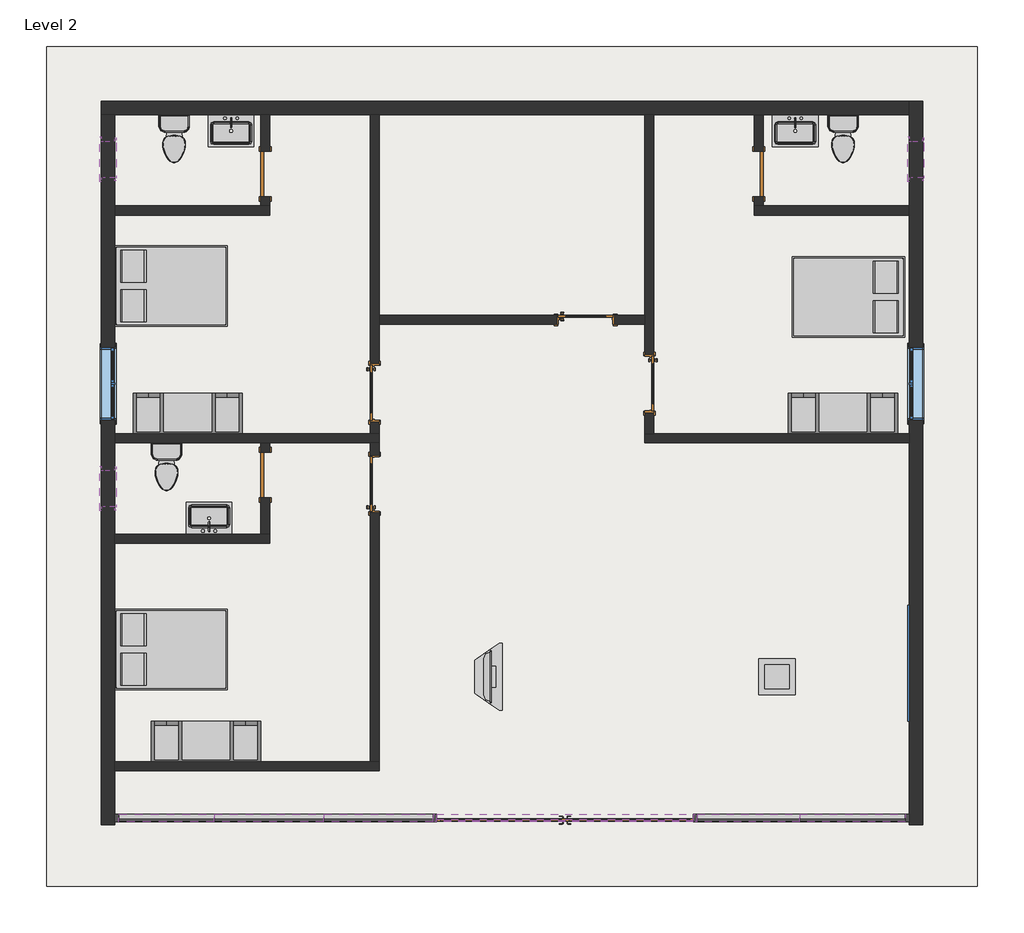
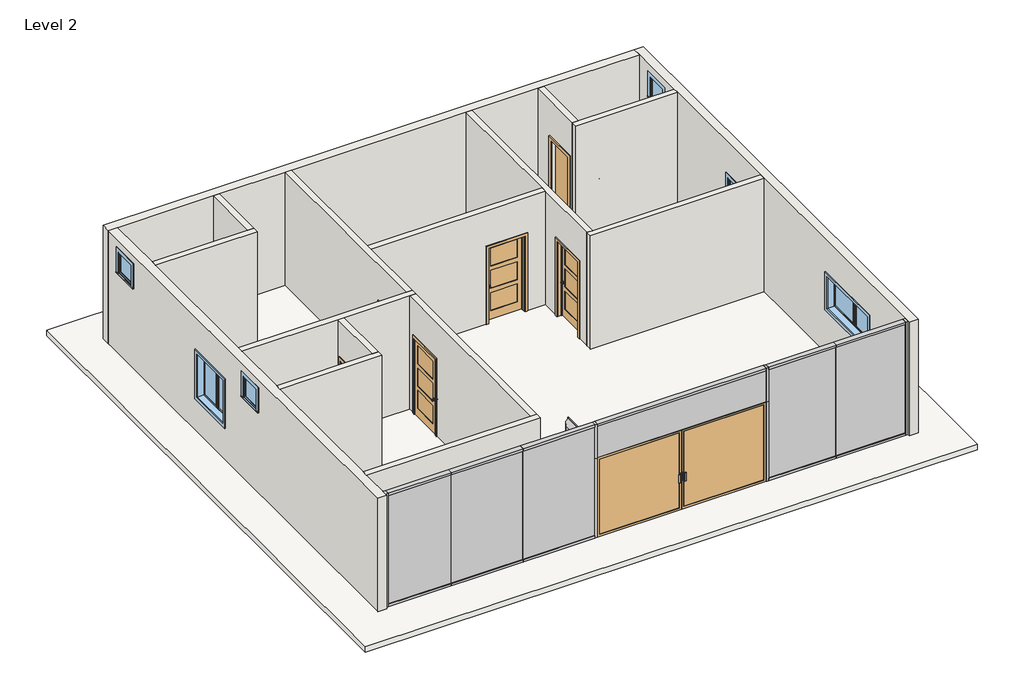
# One storey, incomplete: 17 members, 16 walls, 9 furniture elements, 8 doors, 6 flow terminals, 6 plates, 6 windows, 1 slab.
"""IFC4 building model written with IfcOpenShell, lengths in millimetres."""

from ifc_helpers import new_model, si_unit, frame, origin, place, context, project, spatial, polyline, outline, extrude, faceted_brep, transform, mapped, element, save
from components import door_curtain_wall_double_storefront_door_curtain_wall_double_6e8ba87c, door_ac27962c, door_c5233792, door_d64d7266, door_c31ea698, flow_terminal_38af2918, toilet_domestic_3d_toilet_domestic_3d_f7549cf7, toilet_domestic_3d_toilet_domestic_3d_183bbd19, furniture_c8abb964, furniture_cf0b6580, furniture_56245f3a, tv_stand_tv_stand_94947415, furniture_b5c51a22, member_3f395ae9, member_d9503739, member_2fae0574, member_2501c824, member_6d5c3e5e, member_4da692ab, member_3374d9b6, member_73c23c35, system_panel_glazed_a38948d3, system_panel_glazed_97c7e3fb, system_panel_glazed_baea53c3, system_panel_glazed_5d99744d, system_panel_glazed_41d8189d, window_534dcd48, window_6788402d, window_3ed046d9

model = new_model("IFC4")

# Units and contexts
model_context = context("Model", 3, world=origin())
ifc_project = project(units=[si_unit("LENGTHUNIT", "METRE", prefix="MILLI")], contexts=[model_context])

# Site, building, storey
site = spatial("IfcSite", under=ifc_project)
building = spatial("IfcBuilding", under=site)
storey = spatial("IfcBuildingStorey", under=building, Name="Level 2", Elevation=3048.0)

# Doors
placement = place(None, origin())
door_curtain_wall_double_storefront_door_curtain_wall_double_shape = door_curtain_wall_double_storefront_door_curtain_wall_double_6e8ba87c(model_context)
element("IfcDoor", 1, ObjectType="Door-Curtain-Wall-Double-Storefront : Door-Curtain-Wall-Double-Storefront", at=placement, inside=storey, context=model_context, shape_type="MappedRepresentation", body=[
    mapped(door_curtain_wall_double_storefront_door_curtain_wall_double_shape, transform((-6799.0866603, -9419.3331121, 3048.0), x_axis=(-1.0, 0.0, 0.0), y_axis=(0.0, -1.0, 0.0), z_axis=(0.0, 0.0, 1.0))),
])
door_shape = door_ac27962c(model_context)
element("IfcDoor", 2, ObjectType="Door-Interior-Single-3_Panel_Vert-Wood : 36\" x 80\"", at=placement, inside=storey, context=model_context, shape_type="MappedRepresentation", body=[
    mapped(door_shape, transform((-9989.9616603, -3831.3331121, 3048.0), x_axis=(0.0, 1.0, 0.0), y_axis=(-1.0, 0.0, 0.0), z_axis=(0.0, 0.0, 1.0))),
])
element("IfcDoor", 3, ObjectType="Door-Interior-Single-3_Panel_Vert-Wood : 36\" x 80\"", at=placement, inside=storey, context=model_context, shape_type="MappedRepresentation", body=[
    mapped(door_shape, transform((-5386.2116603, -2154.9331121, 3048.0), x_axis=(0.0, -1.0, 0.0), y_axis=(1.0, 0.0, 0.0), z_axis=(0.0, 0.0, 1.0))),
])
element("IfcDoor", 4, ObjectType="Door-Interior-Single-3_Panel_Vert-Wood : 36\" x 80\"", at=placement, inside=storey, context=model_context, shape_type="MappedRepresentation", body=[
    mapped(door_shape, transform((-6456.1866603, -1084.9581121, 3048.0), x_axis=(1.0, 0.0, 0.0), y_axis=(0.0, 1.0, 0.0), z_axis=(0.0, 0.0, 1.0))),
])
door_2_shape = door_c5233792(model_context)
element("IfcDoor", 5, ObjectType="Door-Interior-Single-3_Panel_Vert-Wood : 36\" x 80\"", at=placement, inside=storey, context=model_context, shape_type="MappedRepresentation", body=[
    mapped(door_2_shape, transform((-9989.9616603, -2307.3331121, 3048.0), x_axis=(0.0, -1.0, 0.0), y_axis=(1.0, 0.0, 0.0), z_axis=(0.0, 0.0, 1.0))),
])
door_3_shape = door_d64d7266(model_context)
element("IfcDoor", 6, ObjectType="Door-Single-Panel : 30\" x 80\"", at=placement, inside=storey, context=model_context, shape_type="MappedRepresentation", body=[
    mapped(door_3_shape, transform((-11815.5866603, 1350.2668879, 3048.0), x_axis=(0.0, -1.0, 0.0), y_axis=(1.0, 0.0, 0.0), z_axis=(0.0, 0.0, 1.0))),
])
door_4_shape = door_c31ea698(model_context)
element("IfcDoor", 7, ObjectType="Door-Single-Panel : 30\" x 80\"", at=placement, inside=storey, context=model_context, shape_type="MappedRepresentation", body=[
    mapped(door_4_shape, transform((-11815.5866603, -3678.9331121, 3048.0), x_axis=(0.0, 1.0, 0.0), y_axis=(-1.0, 0.0, 0.0), z_axis=(0.0, 0.0, 1.0))),
])
element("IfcDoor", 8, ObjectType="Door-Single-Panel : 30\" x 80\"", at=placement, inside=storey, context=model_context, shape_type="MappedRepresentation", body=[
    mapped(door_4_shape, transform((-3560.5866603, 1350.2668879, 3048.0), x_axis=(0.0, -1.0, 0.0), y_axis=(1.0, 0.0, 0.0), z_axis=(0.0, 0.0, 1.0))),
])

# Flow terminals
flow_terminal_shape = flow_terminal_38af2918(model_context)
element("IfcFlowTerminal", 9, ObjectType="Sink Kitchen-Single : 30\" x 21\"", at=placement, inside=storey, context=model_context, shape_type="MappedRepresentation", body=[
    mapped(flow_terminal_shape, transform((-12402.7759008, 2071.8214868, 3048.0), x_axis=(1.0, 0.0, 0.0), y_axis=(0.0, 1.0, 0.0), z_axis=(0.0, 0.0, 1.0))),
])
element("IfcFlowTerminal", 10, ObjectType="Sink Kitchen-Single : 30\" x 21\"", at=placement, inside=storey, context=model_context, shape_type="MappedRepresentation", body=[
    mapped(flow_terminal_shape, transform((-2966.6759008, 2071.8214868, 3048.0), x_axis=(1.0000000000000002, 0.0, 0.0), y_axis=(0.0, 1.0000000000000002, 0.0), z_axis=(0.0, 0.0, 1.0))),
])
element("IfcFlowTerminal", 11, ObjectType="Sink Kitchen-Single : 30\" x 21\"", at=placement, inside=storey, context=model_context, shape_type="MappedRepresentation", body=[
    mapped(flow_terminal_shape, transform((-12739.6974197, -4406.8377109, 3048.0), x_axis=(-1.0000000000000002, 0.0, 0.0), y_axis=(0.0, -1.0000000000000002, 0.0), z_axis=(0.0, 0.0, 1.0))),
])
toilet_domestic_3d_toilet_domestic_3d_shape = toilet_domestic_3d_toilet_domestic_3d_f7549cf7(model_context)
toilet_domestic_3d_toilet_domestic_3d_2_shape = toilet_domestic_3d_toilet_domestic_3d_183bbd19(model_context)
element("IfcFlowTerminal", 12, ObjectType="Toilet-Domestic-3D : Toilet-Domestic-3D", at=placement, inside=storey, context=model_context, shape_type="MappedRepresentation", body=[
    mapped(toilet_domestic_3d_toilet_domestic_3d_shape, transform((-13339.5866603, 1846.1708606, 3048.0), x_axis=(1.0000000000000007, 0.0, 0.0), y_axis=(0.0, 1.0000000000000007, 0.0), z_axis=(0.0, 0.0, 1.0))),
    mapped(toilet_domestic_3d_toilet_domestic_3d_2_shape, transform((-13339.5866603, 1846.1708606, 3048.0), x_axis=(1.0000000000000007, 0.0, 0.0), y_axis=(0.0, 1.0000000000000007, 0.0), z_axis=(0.0, 0.0, 1.0))),
])
element("IfcFlowTerminal", 13, ObjectType="Toilet-Domestic-3D : Toilet-Domestic-3D", at=placement, inside=storey, context=model_context, shape_type="MappedRepresentation", body=[
    mapped(toilet_domestic_3d_toilet_domestic_3d_shape, transform((-2150.8866603, 1846.1708606, 3048.0), x_axis=(1.0, 0.0, 0.0), y_axis=(0.0, 1.0, 0.0), z_axis=(0.0, 0.0, 1.0))),
    mapped(toilet_domestic_3d_toilet_domestic_3d_2_shape, transform((-2150.8866603, 1846.1708606, 3048.0), x_axis=(1.0, 0.0, 0.0), y_axis=(0.0, 1.0, 0.0), z_axis=(0.0, 0.0, 1.0))),
])
element("IfcFlowTerminal", 14, ObjectType="Toilet-Domestic-3D : Toilet-Domestic-3D", at=placement, inside=storey, context=model_context, shape_type="MappedRepresentation", body=[
    mapped(toilet_domestic_3d_toilet_domestic_3d_shape, transform((-13466.5866603, -3640.2291394, 3048.0), x_axis=(1.0, 0.0, 0.0), y_axis=(0.0, 1.0, 0.0), z_axis=(0.0, 0.0, 1.0))),
    mapped(toilet_domestic_3d_toilet_domestic_3d_2_shape, transform((-13466.5866603, -3640.2291394, 3048.0), x_axis=(1.0, 0.0, 0.0), y_axis=(0.0, 1.0, 0.0), z_axis=(0.0, 0.0, 1.0))),
])

# Furniture
furniture_shape = furniture_c8abb964(model_context)
element("IfcFurniture", 15, ObjectType="Bed-Box : Double 53\" x 74\"", at=placement, inside=storey, context=model_context, shape_type="MappedRepresentation", body=[
    mapped(furniture_shape, transform((-13624.8161685, -859.5331121, 3048.0), x_axis=(0.0, 1.0, 0.0), y_axis=(-1.0, 0.0, 0.0), z_axis=(0.0, 0.0, 1.0))),
])
element("IfcFurniture", 16, ObjectType="Bed-Box : Double 53\" x 74\"", at=placement, inside=storey, context=model_context, shape_type="MappedRepresentation", body=[
    mapped(furniture_shape, transform((-13624.8161685, -6939.0855711, 3048.0), x_axis=(0.0, 1.0000000000000002, 0.0), y_axis=(-1.0000000000000002, 0.0, 0.0), z_axis=(0.0, 0.0, 1.0))),
])
element("IfcFurniture", 17, ObjectType="Bed-Box : Double 53\" x 74\"", at=placement, inside=storey, context=model_context, shape_type="MappedRepresentation", body=[
    mapped(furniture_shape, transform((-1827.5571521, -367.980653, 3048.0), x_axis=(0.0, -1.0, 0.0), y_axis=(1.0, 0.0, 0.0), z_axis=(0.0, 0.0, 1.0))),
])
furniture_2_shape = furniture_cf0b6580(model_context)
element("IfcFurniture", 18, ObjectType="Entertainment Center : 72\" x 72\" x 24\"", at=placement, inside=storey, context=model_context, shape_type="MappedRepresentation", body=[
    mapped(furniture_2_shape, transform((-2150.8866603, -3094.7331121, 3048.0), x_axis=(-1.0000000000000002, 0.0, 0.0), y_axis=(0.0, -1.0000000000000002, 0.0), z_axis=(0.0, 0.0, 1.0))),
])
element("IfcFurniture", 19, ObjectType="Entertainment Center : 72\" x 72\" x 24\"", at=placement, inside=storey, context=model_context, shape_type="MappedRepresentation", body=[
    mapped(furniture_2_shape, transform((-13110.9866603, -3094.7331121, 3048.0), x_axis=(-1.0, 0.0, 0.0), y_axis=(0.0, -1.0, 0.0), z_axis=(0.0, 0.0, 1.0))),
])
element("IfcFurniture", 20, ObjectType="Entertainment Center : 72\" x 72\" x 24\"", at=placement, inside=storey, context=model_context, shape_type="MappedRepresentation", body=[
    mapped(furniture_2_shape, transform((-12806.1866603, -8581.1331121, 3048.0), x_axis=(-1.0, 0.0, 0.0), y_axis=(0.0, -1.0, 0.0), z_axis=(0.0, 0.0, 1.0))),
])
furniture_3_shape = furniture_56245f3a(model_context)
element("IfcFurniture", 21, ObjectType="TV - Flat Screen : 32\"", at=placement, inside=storey, context=model_context, shape_type="MappedRepresentation", body=[
    mapped(furniture_3_shape, transform((-8100.8328523, -7053.1885979, 3657.6), x_axis=(0.0, 1.0000000000000002, 0.0), y_axis=(-1.0000000000000002, 0.0, 0.0), z_axis=(0.0, 0.0, 1.0))),
])
tv_stand_tv_stand_shape = tv_stand_tv_stand_94947415(model_context)
element("IfcFurniture", 22, ObjectType="TV Stand : TV Stand", at=placement, inside=storey, context=model_context, shape_type="MappedRepresentation", body=[
    mapped(tv_stand_tv_stand_shape, transform((-8310.3866603, -7182.3211141, 3048.0), x_axis=(0.0, 1.0000000000000002, 0.0), y_axis=(-1.0000000000000002, 0.0, 0.0), z_axis=(0.0, 0.0, 1.0))),
])
furniture_4_shape = furniture_b5c51a22(model_context)
element("IfcFurniture", 23, ObjectType="Table-Coffee : 24\" x 24\" x 24\"", at=placement, inside=storey, context=model_context, shape_type="MappedRepresentation", body=[
    mapped(furniture_4_shape, transform((-3274.0524269, -7152.3441899, 3048.0), x_axis=(1.0, 0.0, 0.0), y_axis=(0.0, 1.0, 0.0), z_axis=(0.0, 0.0, 1.0))),
])

# Members
member_shape = member_3f395ae9(model_context)
element("IfcMember", 24, ObjectType="Rectangular Mullion : 2.5\" x 5\" rectangular", at=placement, inside=storey, context=model_context, shape_type="MappedRepresentation", body=[
    mapped(member_shape, transform((-14330.1866603, -9419.3331121, 3048.0), x_axis=(-1.0, 0.0, 0.0), y_axis=(0.0, 1.0, 0.0), z_axis=(0.0, 0.0, -1.0))),
])
member_2_shape = member_d9503739(model_context)
element("IfcMember", 25, ObjectType="Rectangular Mullion : 2.5\" x 5\" rectangular", at=placement, inside=storey, context=model_context, shape_type="MappedRepresentation", body=[
    mapped(member_2_shape, transform((-14266.6866603, -9419.3331121, 6096.0), x_axis=(0.0, 0.0, 1.0), y_axis=(0.0, 1.0, 0.0), z_axis=(-1.0, 0.0, 0.0))),
])
member_3_shape = member_2fae0574(model_context)
element("IfcMember", 26, ObjectType="Rectangular Mullion : 2.5\" x 5\" rectangular", at=placement, inside=storey, context=model_context, shape_type="MappedRepresentation", body=[
    mapped(member_3_shape, transform((-12666.4866603, -9419.3331121, 6096.0), x_axis=(0.0, 0.0, 1.0), y_axis=(0.0, 1.0, 0.0), z_axis=(-1.0, 0.0, 0.0))),
])
element("IfcMember", 27, ObjectType="Rectangular Mullion : 2.5\" x 5\" rectangular", at=placement, inside=storey, context=model_context, shape_type="MappedRepresentation", body=[
    mapped(member_2_shape, transform((-12666.4866603, -9419.3331121, 3048.0), x_axis=(0.0, 0.0, -1.0), y_axis=(0.0, 1.0, 0.0), z_axis=(1.0, 0.0, 0.0))),
])
element("IfcMember", 28, ObjectType="Rectangular Mullion : 2.5\" x 5\" rectangular", at=placement, inside=storey, context=model_context, shape_type="MappedRepresentation", body=[
    mapped(member_3_shape, transform((-9008.8866603, -9419.3331121, 3048.0), x_axis=(0.0, 0.0, -1.0), y_axis=(0.0, 1.0, 0.0), z_axis=(1.0, 0.0, 0.0))),
])
element("IfcMember", 29, ObjectType="Rectangular Mullion : 2.5\" x 5\" rectangular", at=placement, inside=storey, context=model_context, shape_type="MappedRepresentation", body=[
    mapped(member_3_shape, transform((-10837.6866603, -9419.3331121, 3048.0), x_axis=(0.0, 0.0, -1.0), y_axis=(0.0, 1.0, 0.0), z_axis=(1.0, 0.0, 0.0))),
])
member_4_shape = member_2501c824(model_context)
element("IfcMember", 30, ObjectType="Rectangular Mullion : 2.5\" x 5\" rectangular", at=placement, inside=storey, context=model_context, shape_type="MappedRepresentation", body=[
    mapped(member_4_shape, transform((-2874.7866603, -9419.3331121, 3048.0), x_axis=(0.0, 0.0, -1.0), y_axis=(0.0, 1.0, 0.0), z_axis=(1.0, 0.0, 0.0))),
])
member_5_shape = member_6d5c3e5e(model_context)
element("IfcMember", 31, ObjectType="Rectangular Mullion : 2.5\" x 5\" rectangular", at=placement, inside=storey, context=model_context, shape_type="MappedRepresentation", body=[
    mapped(member_5_shape, transform((-2874.7866603, -9419.3331121, 6096.0), x_axis=(0.0, 0.0, 1.0), y_axis=(0.0, 1.0, 0.0), z_axis=(-1.0, 0.0, 0.0))),
])
element("IfcMember", 32, ObjectType="Rectangular Mullion : 2.5\" x 5\" rectangular", at=placement, inside=storey, context=model_context, shape_type="MappedRepresentation", body=[
    mapped(member_5_shape, transform((-1109.4866603, -9419.3331121, 3048.0), x_axis=(0.0, 0.0, -1.0), y_axis=(0.0, 1.0, 0.0), z_axis=(1.0, 0.0, 0.0))),
])
element("IfcMember", 33, ObjectType="Rectangular Mullion : 2.5\" x 5\" rectangular", at=placement, inside=storey, context=model_context, shape_type="MappedRepresentation", body=[
    mapped(member_shape, transform((-1045.9866603, -9419.3331121, 6096.0), x_axis=(1.0, 0.0, 0.0), y_axis=(0.0, 1.0, 0.0), z_axis=(0.0, 0.0, 1.0))),
])
element("IfcMember", 34, ObjectType="Rectangular Mullion : 2.5\" x 5\" rectangular", at=placement, inside=storey, context=model_context, shape_type="MappedRepresentation", body=[
    mapped(member_3_shape, transform((-10837.6866603, -9419.3331121, 6096.0), x_axis=(0.0, 0.0, 1.0), y_axis=(0.0, 1.0, 0.0), z_axis=(-1.0, 0.0, 0.0))),
])
element("IfcMember", 35, ObjectType="Rectangular Mullion : 2.5\" x 5\" rectangular", at=placement, inside=storey, context=model_context, shape_type="MappedRepresentation", body=[
    mapped(member_4_shape, transform((-4589.2866603, -9419.3331121, 6096.0), x_axis=(0.0, 0.0, 1.0), y_axis=(0.0, 1.0, 0.0), z_axis=(-1.0, 0.0, 0.0))),
])
member_6_shape = member_4da692ab(model_context)
element("IfcMember", 36, ObjectType="Rectangular Mullion : 2.5\" x 5\" rectangular", at=placement, inside=storey, context=model_context, shape_type="MappedRepresentation", body=[
    mapped(member_6_shape, transform((-8945.3866603, -9419.3331121, 6096.0), x_axis=(0.0, 0.0, 1.0), y_axis=(0.0, 1.0, 0.0), z_axis=(-1.0, 0.0, 0.0))),
])
member_7_shape = member_3374d9b6(model_context)
element("IfcMember", 37, ObjectType="Rectangular Mullion : 2.5\" x 5\" rectangular", at=placement, inside=storey, context=model_context, shape_type="MappedRepresentation", body=[
    mapped(member_7_shape, transform((-9008.8866603, -9419.3331121, 3048.0), x_axis=(-1.0, 0.0, 0.0), y_axis=(0.0, 1.0, 0.0), z_axis=(0.0, 0.0, -1.0))),
])
member_8_shape = member_73c23c35(model_context)
element("IfcMember", 38, ObjectType="Rectangular Mullion : 2.5\" x 5\" rectangular", at=placement, inside=storey, context=model_context, shape_type="MappedRepresentation", body=[
    mapped(member_8_shape, transform((-4589.2866603, -9419.3331121, 6096.0), x_axis=(1.0, 0.0, 0.0), y_axis=(0.0, 1.0, 0.0), z_axis=(0.0, 0.0, 1.0))),
])
element("IfcMember", 39, ObjectType="Rectangular Mullion : 2.5\" x 5\" rectangular", at=placement, inside=storey, context=model_context, shape_type="MappedRepresentation", body=[
    mapped(member_8_shape, transform((-9008.8866603, -9419.3331121, 5181.6), x_axis=(-1.0, 0.0, 0.0), y_axis=(0.0, 1.0, 0.0), z_axis=(0.0, 0.0, -1.0))),
])
element("IfcMember", 40, ObjectType="Rectangular Mullion : 2.5\" x 5\" rectangular", at=placement, inside=storey, context=model_context, shape_type="MappedRepresentation", body=[
    mapped(member_7_shape, transform((-4589.2866603, -9419.3331121, 5181.6), x_axis=(1.0, 0.0, 0.0), y_axis=(0.0, 1.0, 0.0), z_axis=(0.0, 0.0, 1.0))),
])

# Plates
system_panel_glazed_shape = system_panel_glazed_a38948d3(model_context)
element("IfcPlate", 41, ObjectType="System Panel : Glazed", at=placement, inside=storey, context=model_context, shape_type="MappedRepresentation", body=[
    mapped(system_panel_glazed_shape, transform((-13466.5866603, -9419.3331121, 3111.5), x_axis=(-1.0, 0.0, 0.0), y_axis=(0.0, -1.0, 0.0), z_axis=(0.0, 0.0, 1.0))),
])
system_panel_glazed_2_shape = system_panel_glazed_97c7e3fb(model_context)
element("IfcPlate", 42, ObjectType="System Panel : Glazed", at=placement, inside=storey, context=model_context, shape_type="MappedRepresentation", body=[
    mapped(system_panel_glazed_2_shape, transform((-9923.2866603, -9419.3331121, 3111.5), x_axis=(-1.0, 0.0, 0.0), y_axis=(0.0, -1.0, 0.0), z_axis=(0.0, 0.0, 1.0))),
])
element("IfcPlate", 43, ObjectType="System Panel : Glazed", at=placement, inside=storey, context=model_context, shape_type="MappedRepresentation", body=[
    mapped(system_panel_glazed_2_shape, transform((-11752.0866603, -9419.3331121, 3111.5), x_axis=(-1.0, 0.0, 0.0), y_axis=(0.0, -1.0, 0.0), z_axis=(0.0, 0.0, 1.0))),
])
system_panel_glazed_3_shape = system_panel_glazed_baea53c3(model_context)
element("IfcPlate", 44, ObjectType="System Panel : Glazed", at=placement, inside=storey, context=model_context, shape_type="MappedRepresentation", body=[
    mapped(system_panel_glazed_3_shape, transform((-3732.0366603, -9419.3331121, 3111.5), x_axis=(-1.0, 0.0, 0.0), y_axis=(0.0, -1.0, 0.0), z_axis=(0.0, 0.0, 1.0))),
])
system_panel_glazed_4_shape = system_panel_glazed_5d99744d(model_context)
element("IfcPlate", 45, ObjectType="System Panel : Glazed", at=placement, inside=storey, context=model_context, shape_type="MappedRepresentation", body=[
    mapped(system_panel_glazed_4_shape, transform((-1992.1366603, -9419.3331121, 3111.5), x_axis=(-1.0, 0.0, 0.0), y_axis=(0.0, -1.0, 0.0), z_axis=(0.0, 0.0, 1.0))),
])
system_panel_glazed_5_shape = system_panel_glazed_41d8189d(model_context)
element("IfcPlate", 46, ObjectType="System Panel : Glazed", at=placement, inside=storey, context=model_context, shape_type="MappedRepresentation", body=[
    mapped(system_panel_glazed_5_shape, transform((-6799.0866603, -9419.3331121, 5181.6), x_axis=(-1.0, 0.0, 0.0), y_axis=(0.0, -1.0, 0.0), z_axis=(0.0, 0.0, 1.0))),
])

# Slab
element("IfcSlab", 47, ObjectType="Generic - 6\" 2", at=placement, inside=storey, context=model_context, shape_type="SweptSolid", body=[
    extrude(outline(polyline([(97.0133397, 3483.8668879), (97.0133397, -10562.3331121), (-15473.1866603, -10562.3331121), (-15473.1866603, 3483.8668879), (97.0133397, 3483.8668879)])), frame((0.0, 0.0, 2895.6), z_axis=(0.0, 0.0, 1.0), x_axis=(1.0, 0.0, 0.0)), (0.0, 0.0, 1.0), 152.4),
])

# Walls
element("IfcWall", 48, ObjectType="Generic - 6\"", at=placement, inside=storey, context=model_context, shape_type="Brep", body=[
    faceted_brep([(-14330.1866603, 664.4668879, 3048.0), (-11739.3866603, 664.4668879, 3048.0), (-11739.3866603, 664.4668879, 6096.0), (-14330.1866603, 664.4668879, 6096.0), (-14330.1866603, 816.8668879, 3048.0), (-14330.1866603, 816.8668879, 6096.0), (-11891.7866603, 816.8668879, 6096.0), (-11739.3866603, 816.8668879, 6096.0), (-11739.3866603, 816.8668879, 3048.0), (-11891.7866603, 816.8668879, 3048.0)], [[[0, 1, 2, 3]], [[4, 5, 6, 7, 8, 9]], [[1, 0, 4, 9, 8]], [[3, 2, 7, 6, 5]], [[0, 3, 5, 4]], [[2, 1, 8, 7]]]),
])
element("IfcWall", 49, ObjectType="Generic - 6\"", at=placement, inside=storey, context=model_context, shape_type="SweptSolid", body=[
    extrude(outline(polyline([(969.2668879, 5080.0), (969.2668879, 3048.0), (816.8668879, 3048.0), (816.8668879, 6096.0), (2340.8668879, 6096.0), (2340.8668879, 3048.0), (1731.2668879, 3048.0), (1731.2668879, 5080.0), (969.2668879, 5080.0)])), frame((-11891.7866603, 0.0, 0.0), z_axis=(1.0, 0.0, 0.0), x_axis=(0.0, 1.0, 0.0)), (0.0, 0.0, 1.0), 152.4),
])
element("IfcWall", 50, ObjectType="Generic - 6\"", at=placement, inside=storey, context=model_context, shape_type="Brep", body=[
    faceted_brep([(-14330.1866603, -3145.5331121, 3048.0), (-11891.7866603, -3145.5331121, 3048.0), (-11739.3866603, -3145.5331121, 3048.0), (-10062.9866603, -3145.5331121, 3048.0), (-9910.5866603, -3145.5331121, 3048.0), (-9910.5866603, -3145.5331121, 6096.0), (-10062.9866603, -3145.5331121, 6096.0), (-11739.3866603, -3145.5331121, 6096.0), (-11891.7866603, -3145.5331121, 6096.0), (-14330.1866603, -3145.5331121, 6096.0), (-14330.1866603, -2993.1331121, 3048.0), (-14330.1866603, -2993.1331121, 6096.0), (-10062.9866603, -2993.1331121, 6096.0), (-9910.5866603, -2993.1331121, 6096.0), (-9910.5866603, -2993.1331121, 3048.0), (-10062.9866603, -2993.1331121, 3048.0)], [[[0, 1, 2, 3, 4, 5, 6, 7, 8, 9]], [[10, 11, 12, 13, 14, 15]], [[4, 3, 2, 1, 0, 10, 15, 14]], [[9, 8, 7, 6, 5, 13, 12, 11]], [[0, 9, 11, 10]], [[5, 4, 14, 13]]]),
])
element("IfcWall", 51, ObjectType="Generic - 6\"", at=placement, inside=storey, context=model_context, shape_type="Brep", body=[
    faceted_brep([(-9910.5866603, 2340.8668879, 6096.0), (-9910.5866603, -1011.9331121, 6096.0), (-9910.5866603, -1164.3331121, 6096.0), (-9910.5866603, -2993.1331121, 6096.0), (-9910.5866603, -2993.1331121, 3048.0), (-9910.5866603, -2789.9331121, 3048.0), (-9910.5866603, -2789.9331121, 5105.4), (-9910.5866603, -1824.7331121, 5105.4), (-9910.5866603, -1824.7331121, 3048.0), (-9910.5866603, -1164.3331121, 3048.0), (-9910.5866603, -1011.9331121, 3048.0), (-9910.5866603, 2340.8668879, 3048.0), (-10062.9866603, -2993.1331121, 6096.0), (-10062.9866603, 2340.8668879, 6096.0), (-10062.9866603, 2340.8668879, 3048.0), (-10062.9866603, -1824.7331121, 3048.0), (-10062.9866603, -1824.7331121, 5105.4), (-10062.9866603, -2789.9331121, 5105.4), (-10062.9866603, -2789.9331121, 3048.0), (-10062.9866603, -2993.1331121, 3048.0)], [[[0, 1, 2, 3, 4, 5, 6, 7, 8, 9, 10, 11]], [[12, 13, 14, 15, 16, 17, 18, 19]], [[4, 19, 18, 5]], [[14, 11, 10, 9, 8, 15]], [[3, 2, 1, 0, 13, 12]], [[4, 3, 12, 19]], [[0, 11, 14, 13]], [[17, 6, 5, 18]], [[6, 17, 16, 7]], [[7, 16, 15, 8]]]),
])
element("IfcWall", 52, ObjectType="Generic - 6\"", at=placement, inside=storey, context=model_context, shape_type="Brep", body=[
    faceted_brep([(-14330.1866603, -4821.9331121, 3048.0), (-11739.3866603, -4821.9331121, 3048.0), (-11739.3866603, -4821.9331121, 6096.0), (-14330.1866603, -4821.9331121, 6096.0), (-14330.1866603, -4669.5331121, 3048.0), (-14330.1866603, -4669.5331121, 6096.0), (-11891.7866603, -4669.5331121, 6096.0), (-11739.3866603, -4669.5331121, 6096.0), (-11739.3866603, -4669.5331121, 3048.0), (-11891.7866603, -4669.5331121, 3048.0)], [[[0, 1, 2, 3]], [[4, 5, 6, 7, 8, 9]], [[1, 0, 4, 9, 8]], [[3, 2, 7, 6, 5]], [[2, 1, 8, 7]], [[0, 3, 5, 4]]]),
])
element("IfcWall", 53, ObjectType="Generic - 6\"", at=placement, inside=storey, context=model_context, shape_type="SweptSolid", body=[
    extrude(outline(polyline([(-3145.5331121, 3048.0), (-3297.9331121, 3048.0), (-3297.9331121, 5080.0), (-4059.9331121, 5080.0), (-4059.9331121, 3048.0), (-4669.5331121, 3048.0), (-4669.5331121, 6096.0), (-3145.5331121, 6096.0), (-3145.5331121, 3048.0)])), frame((-11891.7866603, 0.0, 0.0), z_axis=(1.0, 0.0, 0.0), x_axis=(0.0, 1.0, 0.0)), (0.0, 0.0, 1.0), 152.4),
])
element("IfcWall", 54, ObjectType="Generic - 6\"", at=placement, inside=storey, context=model_context, shape_type="Brep", body=[
    faceted_brep([(-14330.1866603, -8631.9331121, 3048.0), (-9910.5866603, -8631.9331121, 3048.0), (-9910.5866603, -8631.9331121, 6096.0), (-14330.1866603, -8631.9331121, 6096.0), (-14330.1866603, -8479.5331121, 3048.0), (-14330.1866603, -8479.5331121, 6096.0), (-10062.9866603, -8479.5331121, 6096.0), (-9910.5866603, -8479.5331121, 6096.0), (-9910.5866603, -8479.5331121, 3048.0), (-10062.9866603, -8479.5331121, 3048.0)], [[[0, 1, 2, 3]], [[4, 5, 6, 7, 8, 9]], [[1, 0, 4, 9, 8]], [[3, 2, 7, 6, 5]], [[2, 1, 8, 7]], [[0, 3, 5, 4]]]),
])
element("IfcWall", 55, ObjectType="Generic - 6\"", at=placement, inside=storey, context=model_context, shape_type="SweptSolid", body=[
    extrude(outline(polyline([(-8479.5331121, 6096.0), (-3145.5331121, 6096.0), (-3145.5331121, 3048.0), (-3348.7331121, 3048.0), (-3348.7331121, 5105.4), (-4313.9331121, 5105.4), (-4313.9331121, 3048.0), (-8479.5331121, 3048.0), (-8479.5331121, 6096.0)])), frame((-10062.9866603, 0.0, 0.0), z_axis=(1.0, 0.0, 0.0), x_axis=(0.0, 1.0, 0.0)), (0.0, 0.0, 1.0), 152.4),
])
element("IfcWall", 56, ObjectType="Generic - 6\"", at=placement, inside=storey, context=model_context, shape_type="Brep", body=[
    faceted_brep([(-1045.9866603, 816.8668879, 3048.0), (-3484.3866603, 816.8668879, 3048.0), (-3636.7866603, 816.8668879, 3048.0), (-3636.7866603, 816.8668879, 6096.0), (-3484.3866603, 816.8668879, 6096.0), (-1045.9866603, 816.8668879, 6096.0), (-1045.9866603, 664.4668879, 3048.0), (-1045.9866603, 664.4668879, 6096.0), (-3636.7866603, 664.4668879, 6096.0), (-3636.7866603, 664.4668879, 3048.0)], [[[0, 1, 2, 3, 4, 5]], [[6, 7, 8, 9]], [[2, 1, 0, 6, 9]], [[5, 4, 3, 8, 7]], [[0, 5, 7, 6]], [[3, 2, 9, 8]]]),
])
element("IfcWall", 57, ObjectType="Generic - 6\"", at=placement, inside=storey, context=model_context, shape_type="SweptSolid", body=[
    extrude(outline(polyline([(969.2668879, 5080.0), (969.2668879, 3048.0), (816.8668879, 3048.0), (816.8668879, 6096.0), (2340.8668879, 6096.0), (2340.8668879, 3048.0), (1731.2668879, 3048.0), (1731.2668879, 5080.0), (969.2668879, 5080.0)])), frame((-3636.7866603, 0.0, 0.0), z_axis=(1.0, 0.0, 0.0), x_axis=(0.0, 1.0, 0.0)), (0.0, 0.0, 1.0), 152.4),
])
element("IfcWall", 58, ObjectType="Generic - 6\"", at=placement, inside=storey, context=model_context, shape_type="Brep", body=[
    faceted_brep([(-1045.9866603, -2993.1331121, 3048.0), (-5313.1866603, -2993.1331121, 3048.0), (-5465.5866603, -2993.1331121, 3048.0), (-5465.5866603, -2993.1331121, 6096.0), (-5313.1866603, -2993.1331121, 6096.0), (-1045.9866603, -2993.1331121, 6096.0), (-1045.9866603, -3145.5331121, 3048.0), (-1045.9866603, -3145.5331121, 6096.0), (-5465.5866603, -3145.5331121, 6096.0), (-5465.5866603, -3145.5331121, 3048.0)], [[[0, 1, 2, 3, 4, 5]], [[6, 7, 8, 9]], [[2, 1, 0, 6, 9]], [[5, 4, 3, 8, 7]], [[0, 5, 7, 6]], [[3, 2, 9, 8]]]),
])
element("IfcWall", 59, ObjectType="Generic - 6\"", at=placement, inside=storey, context=model_context, shape_type="Brep", body=[
    faceted_brep([(-5313.1866603, 2340.8668879, 6096.0), (-5313.1866603, -2993.1331121, 6096.0), (-5313.1866603, -2993.1331121, 3048.0), (-5313.1866603, -2637.5331121, 3048.0), (-5313.1866603, -2637.5331121, 5105.4), (-5313.1866603, -1672.3331121, 5105.4), (-5313.1866603, -1672.3331121, 3048.0), (-5313.1866603, 2340.8668879, 3048.0), (-5465.5866603, -2993.1331121, 6096.0), (-5465.5866603, -1164.3331121, 6096.0), (-5465.5866603, -1011.9331121, 6096.0), (-5465.5866603, 2340.8668879, 6096.0), (-5465.5866603, 2340.8668879, 3048.0), (-5465.5866603, -1011.9331121, 3048.0), (-5465.5866603, -1164.3331121, 3048.0), (-5465.5866603, -1672.3331121, 3048.0), (-5465.5866603, -1672.3331121, 5105.4), (-5465.5866603, -2637.5331121, 5105.4), (-5465.5866603, -2637.5331121, 3048.0), (-5465.5866603, -2993.1331121, 3048.0)], [[[0, 1, 2, 3, 4, 5, 6, 7]], [[8, 9, 10, 11, 12, 13, 14, 15, 16, 17, 18, 19]], [[2, 19, 18, 3]], [[12, 7, 6, 15, 14, 13]], [[1, 0, 11, 10, 9, 8]], [[2, 1, 8, 19]], [[0, 7, 12, 11]], [[17, 4, 3, 18]], [[4, 17, 16, 5]], [[5, 16, 15, 6]]]),
])
element("IfcWall", 60, ObjectType="Generic - 6\"", at=placement, inside=storey, context=model_context, shape_type="SweptSolid", body=[
    extrude(outline(polyline([(6096.0, -5465.5866603), (6096.0, -9910.5866603), (3048.0, -9910.5866603), (3048.0, -6938.7866603), (5105.4, -6938.7866603), (5105.4, -5973.5866603), (3048.0, -5973.5866603), (3048.0, -5465.5866603), (6096.0, -5465.5866603)])), frame((0.0, -1164.3331121, 0.0), z_axis=(0.0, 1.0, 0.0), x_axis=(0.0, 0.0, 1.0)), (0.0, 0.0, 1.0), 152.4),
])
element("IfcWall", 61, ObjectType="Generic - 9\" 2", at=placement, inside=storey, context=model_context, shape_type="Brep", body=[
    faceted_brep([(-14558.7866603, 2340.8668879, 3048.0), (-14330.1866603, 2340.8668879, 3048.0), (-11891.7866603, 2340.8668879, 3048.0), (-11739.3866603, 2340.8668879, 3048.0), (-10062.9866603, 2340.8668879, 3048.0), (-9910.5866603, 2340.8668879, 3048.0), (-5465.5866603, 2340.8668879, 3048.0), (-5313.1866603, 2340.8668879, 3048.0), (-3636.7866603, 2340.8668879, 3048.0), (-3484.3866603, 2340.8668879, 3048.0), (-1045.9866603, 2340.8668879, 3048.0), (-1045.9866603, 2340.8668879, 6096.0), (-3484.3866603, 2340.8668879, 6096.0), (-3636.7866603, 2340.8668879, 6096.0), (-5313.1866603, 2340.8668879, 6096.0), (-5465.5866603, 2340.8668879, 6096.0), (-9910.5866603, 2340.8668879, 6096.0), (-10062.9866603, 2340.8668879, 6096.0), (-11739.3866603, 2340.8668879, 6096.0), (-11891.7866603, 2340.8668879, 6096.0), (-14330.1866603, 2340.8668879, 6096.0), (-14558.7866603, 2340.8668879, 6096.0), (-14558.7866603, 2569.4668879, 3048.0), (-14558.7866603, 2569.4668879, 6096.0), (-1045.9866603, 2569.4668879, 6096.0), (-1045.9866603, 2569.4668879, 3048.0)], [[[0, 1, 2, 3, 4, 5, 6, 7, 8, 9, 10, 11, 12, 13, 14, 15, 16, 17, 18, 19, 20, 21]], [[22, 23, 24, 25]], [[10, 9, 8, 7, 6, 5, 4, 3, 2, 1, 0, 22, 25]], [[21, 20, 19, 18, 17, 16, 15, 14, 13, 12, 11, 24, 23]], [[0, 21, 23, 22]], [[11, 10, 25, 24]]]),
])
element("IfcWall", 62, ObjectType="Generic - 9\" 2", at=placement, inside=storey, context=model_context, shape_type="Brep", body=[
    faceted_brep([(-14330.1866603, -9533.6331121, 3048.0), (-14330.1866603, -8631.9331121, 3048.0), (-14330.1866603, -8479.5331121, 3048.0), (-14330.1866603, -4821.9331121, 3048.0), (-14330.1866603, -4669.5331121, 3048.0), (-14330.1866603, -3145.5331121, 3048.0), (-14330.1866603, -2993.1331121, 3048.0), (-14330.1866603, 664.4668879, 3048.0), (-14330.1866603, 816.8668879, 3048.0), (-14330.1866603, 2340.8668879, 3048.0), (-14330.1866603, 2340.8668879, 6096.0), (-14330.1866603, 816.8668879, 6096.0), (-14330.1866603, 664.4668879, 6096.0), (-14330.1866603, -2993.1331121, 6096.0), (-14330.1866603, -3145.5331121, 6096.0), (-14330.1866603, -4669.5331121, 6096.0), (-14330.1866603, -4821.9331121, 6096.0), (-14330.1866603, -8479.5331121, 6096.0), (-14330.1866603, -8631.9331121, 6096.0), (-14330.1866603, -9533.6331121, 6096.0), (-14330.1866603, -3602.7331121, 5816.6), (-14330.1866603, -3602.7331121, 5207.0), (-14330.1866603, -4212.3331121, 5207.0), (-14330.1866603, -4212.3331121, 5816.6), (-14330.1866603, 1902.7168879, 5816.6), (-14330.1866603, 1902.7168879, 5207.0), (-14330.1866603, 1293.1168879, 5207.0), (-14330.1866603, 1293.1168879, 5816.6), (-14330.1866603, -2764.5331121, 5181.6), (-14330.1866603, -1545.3331121, 5181.6), (-14330.1866603, -1545.3331121, 3962.4), (-14330.1866603, -2764.5331121, 3962.4), (-14558.7866603, -9533.6331121, 3048.0), (-14558.7866603, -9533.6331121, 6096.0), (-14558.7866603, 2340.8668879, 6096.0), (-14558.7866603, 2340.8668879, 3048.0), (-14558.7866603, -3602.7331121, 5816.6), (-14558.7866603, -4212.3331121, 5816.6), (-14558.7866603, -4212.3331121, 5207.0), (-14558.7866603, -3602.7331121, 5207.0), (-14558.7866603, 1902.7168879, 5816.6), (-14558.7866603, 1293.1168879, 5816.6), (-14558.7866603, 1293.1168879, 5207.0), (-14558.7866603, 1902.7168879, 5207.0), (-14558.7866603, -2764.5331121, 5181.6), (-14558.7866603, -2764.5331121, 3962.4), (-14558.7866603, -1545.3331121, 3962.4), (-14558.7866603, -1545.3331121, 5181.6)], [[[0, 1, 2, 3, 4, 5, 6, 7, 8, 9, 10, 11, 12, 13, 14, 15, 16, 17, 18, 19], [20, 21, 22, 23], [24, 25, 26, 27], [28, 29, 30, 31]], [[32, 33, 34, 35], [36, 37, 38, 39], [40, 41, 42, 43], [44, 45, 46, 47]], [[9, 8, 7, 6, 5, 4, 3, 2, 1, 0, 32, 35]], [[19, 18, 17, 16, 15, 14, 13, 12, 11, 10, 34, 33]], [[0, 19, 33, 32]], [[10, 9, 35, 34]], [[21, 20, 36, 39]], [[22, 21, 39, 38]], [[23, 22, 38, 37]], [[20, 23, 37, 36]], [[25, 24, 40, 43]], [[26, 25, 43, 42]], [[27, 26, 42, 41]], [[24, 27, 41, 40]], [[45, 44, 28, 31]], [[46, 45, 31, 30]], [[47, 46, 30, 29]], [[44, 47, 29, 28]]]),
])
element("IfcWall", 63, ObjectType="Generic - 9\" 2", at=placement, inside=storey, context=model_context, shape_type="Brep", body=[
    faceted_brep([(-1045.9866603, 2569.4668879, 3048.0), (-1045.9866603, 2340.8668879, 3048.0), (-1045.9866603, 816.8668879, 3048.0), (-1045.9866603, 664.4668879, 3048.0), (-1045.9866603, -2993.1331121, 3048.0), (-1045.9866603, -3145.5331121, 3048.0), (-1045.9866603, -9533.6331121, 3048.0), (-1045.9866603, -9533.6331121, 6096.0), (-1045.9866603, -3145.5331121, 6096.0), (-1045.9866603, -2993.1331121, 6096.0), (-1045.9866603, 664.4668879, 6096.0), (-1045.9866603, 816.8668879, 6096.0), (-1045.9866603, 2340.8668879, 6096.0), (-1045.9866603, 2569.4668879, 6096.0), (-1045.9866603, 1902.7168879, 5816.6), (-1045.9866603, 1293.1168879, 5816.6), (-1045.9866603, 1293.1168879, 5207.0), (-1045.9866603, 1902.7168879, 5207.0), (-1045.9866603, -1545.3331121, 5181.6), (-1045.9866603, -2764.5331121, 5181.6), (-1045.9866603, -2764.5331121, 3962.4), (-1045.9866603, -1545.3331121, 3962.4), (-1045.9866603, -7742.9331121, 5181.6), (-1045.9866603, -7742.9331121, 4267.2), (-1045.9866603, -5914.1331121, 4267.2), (-1045.9866603, -5914.1331121, 5181.6), (-817.3866603, 2569.4668879, 3048.0), (-817.3866603, 2569.4668879, 6096.0), (-817.3866603, -9533.6331121, 6096.0), (-817.3866603, -9533.6331121, 3048.0), (-817.3866603, 1902.7168879, 5816.6), (-817.3866603, 1902.7168879, 5207.0), (-817.3866603, 1293.1168879, 5207.0), (-817.3866603, 1293.1168879, 5816.6), (-817.3866603, -1545.3331121, 5181.6), (-817.3866603, -1545.3331121, 3962.4), (-817.3866603, -2764.5331121, 3962.4), (-817.3866603, -2764.5331121, 5181.6), (-817.3866603, -7742.9331121, 5181.6), (-817.3866603, -5914.1331121, 5181.6), (-817.3866603, -5914.1331121, 4267.2), (-817.3866603, -7742.9331121, 4267.2)], [[[0, 1, 2, 3, 4, 5, 6, 7, 8, 9, 10, 11, 12, 13], [14, 15, 16, 17], [18, 19, 20, 21], [22, 23, 24, 25]], [[26, 27, 28, 29], [30, 31, 32, 33], [34, 35, 36, 37], [38, 39, 40, 41]], [[6, 5, 4, 3, 2, 1, 0, 26, 29]], [[7, 6, 29, 28]], [[13, 12, 11, 10, 9, 8, 7, 28, 27]], [[0, 13, 27, 26]], [[31, 30, 14, 17]], [[32, 31, 17, 16]], [[33, 32, 16, 15]], [[30, 33, 15, 14]], [[35, 34, 18, 21]], [[36, 35, 21, 20]], [[37, 36, 20, 19]], [[34, 37, 19, 18]], [[23, 22, 38, 41]], [[24, 23, 41, 40]], [[25, 24, 40, 39]], [[22, 25, 39, 38]]]),
])

# Windows
window_shape = window_534dcd48(model_context)
element("IfcWindow", 64, ObjectType="Casement Dbl with Trim : 48\" x 48\"", at=placement, inside=storey, context=model_context, shape_type="MappedRepresentation", body=[
    mapped(window_shape, transform((-14463.5366603, -2154.9331121, 3048.0), x_axis=(0.0, -1.0, 0.0), y_axis=(1.0, 0.0, 0.0), z_axis=(0.0, 0.0, 1.0))),
])
element("IfcWindow", 65, ObjectType="Casement Dbl with Trim : 48\" x 48\"", at=placement, inside=storey, context=model_context, shape_type="MappedRepresentation", body=[
    mapped(window_shape, transform((-912.6366603, -2154.9331121, 3048.0), x_axis=(0.0, 1.0, 0.0), y_axis=(-1.0, 0.0, 0.0), z_axis=(0.0, 0.0, 1.0))),
])
window_2_shape = window_6788402d(model_context)
element("IfcWindow", 66, ObjectType="Casement Dbl with Trim : 72\" x 36\"", at=placement, inside=storey, context=model_context, shape_type="MappedRepresentation", body=[
    mapped(window_2_shape, transform((-950.7366603, -6828.5331121, 3048.0), x_axis=(0.0, -1.0, 0.0), y_axis=(1.0, 0.0, 0.0), z_axis=(0.0, 0.0, 1.0))),
])
window_3_shape = window_3ed046d9(model_context)
element("IfcWindow", 67, ObjectType="Transom with Trim : 24\" x 24\"", at=placement, inside=storey, context=model_context, shape_type="MappedRepresentation", body=[
    mapped(window_3_shape, transform((-14444.4866603, -3869.4331121, 3048.0), x_axis=(0.0, 1.0, 0.0), y_axis=(-1.0, 0.0, 0.0), z_axis=(0.0, 0.0, 1.0))),
])
element("IfcWindow", 68, ObjectType="Transom with Trim : 24\" x 24\"", at=placement, inside=storey, context=model_context, shape_type="MappedRepresentation", body=[
    mapped(window_3_shape, transform((-14444.4866603, 1636.0168879, 3048.0), x_axis=(0.0, 1.0, 0.0), y_axis=(-1.0, 0.0, 0.0), z_axis=(0.0, 0.0, 1.0))),
])
element("IfcWindow", 69, ObjectType="Transom with Trim : 24\" x 24\"", at=placement, inside=storey, context=model_context, shape_type="MappedRepresentation", body=[
    mapped(window_3_shape, transform((-931.6866603, 1636.0168879, 3048.0), x_axis=(0.0, 1.0, 0.0), y_axis=(-1.0, 0.0, 0.0), z_axis=(0.0, 0.0, 1.0))),
])

save(model, "model.ifc")

# Revit data of these elements
# Type "Door-Curtain-Wall-Double-Storefront : Door-Curtain-Wall-Double-Storefront"
#   Type Mark = "14"
#   Construction Type Id = "opn-d46"
#   Assembly Code = "B2030100"
#   Analytic Construction = "Metal frame, double glass door"
#   Width [instance default] = 6' - 0"
#   Thermal Resistance (R) = 1.3794 (h·ft²·°F)/BTU
#   Swing Angle [instance default] = 90.00°
#   Panel Width [instance default] = 3' - 0"
#   Offset = 0' - 2 1/4"
#   Heat Transfer Coefficient (U) = 0.7250 BTU/(h·ft²·°F)
#   Define Thermal Properties by = 1
#   Function = 1
#   Frame Material = Aluminum
#   Door Handle Material = Aluminum
#   Glazing = Glass
#   Visual Light Transmittance = 0
#   Solar Heat Gain Coefficient = 0
# Type "Door-Interior-Single-3_Panel_Vert-Wood : 36\" x 80\""
#   Type Mark = "10"
#   Assembly Code = "C1020300"
#   Analytic Construction = "Wooden"
#   Top Rail = 0' - 4 11/16"
#   Thickness = 0' - 1 3/8"
#   Thermal Resistance (R) = 2.5876 (h·ft²·°F)/BTU
#   Swing Angle [instance default] = 90.00°
#   Stiles = 0' - 4 3/4"
#   Rough Width = 3' - 2"
#   Rough Height = 6' - 9"
#   Intermediate Rail = 0' - 4 1/2"
#   Height = 6' - 8"
#   Width = 3' - 0"
#   Heat Transfer Coefficient (U) = 0.3865 BTU/(h·ft²·°F)
#   Bottom Rail = 0' - 9 1/8"
#   Trim Material = Cherry
#   Panel Material = Cherry
#   Frame Material = Cherry
#   Door Handle Material = Aluminum
#   Visual Light Transmittance = 0
#   Solar Heat Gain Coefficient = 0
#   Wall Closure = (empty or 0)
#   Function = (empty or 0)
# Type "Door-Single-Panel : 30\" x 80\""
#   Type Mark = "11"
#   Construction Type Id = "DOOR"
#   Assembly Code = "C1020300"
#   Analytic Construction = "Wooden"
#   Thickness = 0' - 2"
#   Thermal Resistance (R) = 2.5876 (h·ft²·°F)/BTU
#   Swing Angle [instance default] = 90.00°
#   Heat Transfer Coefficient (U) = 0.3865 BTU/(h·ft²·°F)
#   Height = 6' - 8"
#   Trim Projection Ext = 0' - 1"
#   Trim Projection Int = 0' - 1"
#   Trim Width = 0' - 3"
#   Width = 2' - 6"
#   Define Thermal Properties by = 1
#   Panel Material = Wood - Birch - Solid Stained Light Low Gloss
#   Trim Material = Paint - Sienna
#   Visual Light Transmittance = 0
#   Solar Heat Gain Coefficient = 0
#   Function = (empty or 0)
#   Wall Closure = (empty or 0)
# Type "Sink Kitchen-Single : 30\" x 21\""
#   Assembly Code = "D2010410"
#   Counter Height = 3' - 0"
#   Depth = 1' - 9"
#   Width = 2' - 6"
#   Faucet Material = Steel, Polished
#   Sink Material = Steel, Polished
#   Default Elevation = 0
# Type "Toilet-Domestic-3D : Toilet-Domestic-3D"
#   Assembly Code = "D2010110"
#   Toilet - Bowl/Basin Material = Porcelain, Linen
#   Toilet - Seat Material = Laminate, Linen, Matte
#   Default Elevation = 0
# Type "Bed-Box : Double 53\" x 74\""
#   Assembly Code = "E2020200"
#   Length = 6' - 2"
#   Width = 4' - 5"
#   Frame Material = Birch
#   Mattress Material = Linen, White
#   Default Elevation = 0
# Type "Entertainment Center : 72\" x 72\" x 24\""
#   Assembly Code = "E2020200"
#   Center Width = 2' - 8"
#   Depth = 2' - 0"
#   Height = 6' - 0"
#   Width = 6' - 0"
#   Material = none
#   Default Elevation = 0
# Type "TV - Flat Screen : 32\""
#   SinAng = 0' - 0.0193"
#   L = 2' - 3.79372"
#   H = 1' - 3.6354"
#   Thickness = 0' - 4.33071"
#   Diagonal = 2' - 7.88976"
#   CosAng = 0' - 0.03431"
#   Stand [instance default] = yes
#   Default Elevation = 0
# Type "TV Stand : TV Stand"
#   Depth = 1' - 6"
#   Width = 3' - 8"
#   Height = 2' - 0"
#   Finish = Melamine - Gray
#   Default Elevation = 0
# Type "Table-Coffee : 24\" x 24\" x 24\""
#   Assembly Code = "E2020200"
#   Height = 2' - 0"
#   Length = 2' - 0"
#   Width = 2' - 0"
#   Top Material = none
#   Frame Material = none
#   Default Elevation = 0
# Type "Rectangular Mullion : 2.5\" x 5\" rectangular"
#   built-in parameter 1007304 = 0.416667 (stored number, unit not read)
#   built-in parameter 1007301 = 0.104167 (stored number, unit not read)
#   built-in parameter 1007300 = 0.104167 (stored number, unit not read)
# Type "System Panel : Glazed"
#   Construction Type Id = "GSP4R"
#   Analytic Construction = "1/8 in Pilkington single glazing"
#   Visual Light Transmittance = 0.9
#   Solar Heat Gain Coefficient = 0.86
#   Heat Transfer Coefficient (U) = 1.18115 BTU/(h·ft²·°F)
# Type "Generic - 6\" 2"
#   Assembly Code = "B1010"
#   Function = 0
#   Layers, outside or top first: 0' - 6" no material (function 1)
# Type "Generic - 6\""
#   Assembly Code = "B2010"
#   Layers, outside or top first: 0' - 6" no material (function 1)
# Type "Generic - 9\" 2"
#   Assembly Code = "B2010"
#   Layers, outside or top first: 0' - 9" no material (function 1)
# Type "Casement Dbl with Trim : 48\" x 48\""
#   Type Mark = "10"
#   Construction Type Id = "GSP4R"
#   Assembly Code = "B2020100"
#   Analytic Construction = "1/8 in Pilkington single glazing"
#   Visual Light Transmittance = 0.9
#   Solar Heat Gain Coefficient = 0.78
#   Heat Transfer Coefficient (U) = 0.6496 BTU/(h·ft²·°F)
#   Height = 4' - 0"
#   Default Sill Height = 3' - 0"
#   Trim Projection - Ext. = 0' - 0 1/2"
#   Trim Projection - Int. = 0' - 0 3/4"
#   Trim Width - Exterior = 0' - 3 1/2"
#   Trim Width - Interior = 0' - 3 1/2"
#   Width = 4' - 0"
#   Window Inset = 0' - 0 3/4"
#   Define Thermal Properties by = 1
#   Glass Pane Material = Glass
#   Sash Material = Sash
#   Trim Exterior Material = Trim
#   Trim Interior Material = Trim
#   Wall Closure = (empty or 0)
# Type "Casement Dbl with Trim : 72\" x 36\""
#   Type Mark = "11"
#   Construction Type Id = "GSP4R"
#   Assembly Code = "B2020100"
#   Analytic Construction = "1/8 in Pilkington single glazing"
#   Visual Light Transmittance = 0.9
#   Solar Heat Gain Coefficient = 0.78
#   Heat Transfer Coefficient (U) = 0.6496 BTU/(h·ft²·°F)
#   Height = 3' - 0"
#   Default Sill Height = 4' - 0"
#   Trim Projection - Ext. = 0' - 0 1/2"
#   Trim Projection - Int. = 0' - 0 3/4"
#   Trim Width - Exterior = 0' - 3 1/2"
#   Trim Width - Interior = 0' - 3 1/2"
#   Width = 6' - 0"
#   Window Inset = 0' - 0 3/4"
#   Define Thermal Properties by = 1
#   Glass Pane Material = Glass
#   Sash Material = Sash
#   Trim Exterior Material = Trim
#   Trim Interior Material = Trim
#   Wall Closure = (empty or 0)
# Type "Transom with Trim : 24\" x 24\""
#   Type Mark = "13"
#   Construction Type Id = "GSP4R"
#   Assembly Code = "B2020100"
#   Analytic Construction = "1/8 in Pilkington single glazing"
#   Visual Light Transmittance = 0.9
#   Solar Heat Gain Coefficient = 0.78
#   Heat Transfer Coefficient (U) = 0.6496 BTU/(h·ft²·°F)
#   Height = 2' - 0"
#   Default Sill Height = 7' - 1"
#   Trim Projection - Ext. = 0' - 0 1/2"
#   Trim Projection - Int. = 0' - 0 3/4"
#   Trim Width - Exterior = 0' - 3 1/2"
#   Trim Width - Interior = 0' - 3 1/2"
#   Width = 2' - 0"
#   Window Inset = 0' - 0 3/4"
#   Define Thermal Properties by = 1
#   Glass Pane Material = Glass
#   Sash Material = Sash
#   Trim Exterior Material = Trim
#   Trim Interior Material = Trim
#   Wall Closure = (empty or 0)
# Element 1 (IfcDoor, "Door-Curtain-Wall-Double-Storefront : Door-Curtain-Wall-Double-Storefront")
#   Swing Angle = 90.00°
#   Phase Created = New Construction
#   Materials on its faces: "Aluminum", "Glass"
# Elements 2, 3, 4, 5 (IfcDoor, "Door-Interior-Single-3_Panel_Vert-Wood : 36\" x 80\"")
#   Swing Angle = 90.00°
#   Phase Created = New Construction
#   Materials on its faces: "Cherry", "Aluminum"
# Elements 6, 7, 8 (IfcDoor, "Door-Single-Panel : 30\" x 80\"")
#   Swing Angle = 90.00°
#   Phase Created = New Construction
#   Materials on its faces: "Paint - Sienna", "Wood - Birch - Solid Stained Light Low Gloss"
# Element 9 (IfcFlowTerminal, "Sink Kitchen-Single : 30\" x 21\"")
#   Mark = "6"
#   Phase Created = New Construction
#   Materials on its faces: "Steel, Polished"
# Element 10 (IfcFlowTerminal, "Sink Kitchen-Single : 30\" x 21\"")
#   Mark = "7"
#   Phase Created = New Construction
#   Materials on its faces: "Steel, Polished"
# Element 11 (IfcFlowTerminal, "Sink Kitchen-Single : 30\" x 21\"")
#   Mark = "8"
#   Phase Created = New Construction
#   Materials on its faces: "Steel, Polished"
# Element 12 (IfcFlowTerminal, "Toilet-Domestic-3D : Toilet-Domestic-3D")
#   Mark = "3"
#   Phase Created = New Construction
#   Materials on its faces: "Porcelain, Linen", "Laminate, Linen, Matte"
# Element 13 (IfcFlowTerminal, "Toilet-Domestic-3D : Toilet-Domestic-3D")
#   Mark = "4"
#   Phase Created = New Construction
#   Materials on its faces: "Porcelain, Linen", "Laminate, Linen, Matte"
# Element 14 (IfcFlowTerminal, "Toilet-Domestic-3D : Toilet-Domestic-3D")
#   Mark = "5"
#   Phase Created = New Construction
#   Materials on its faces: "Porcelain, Linen", "Laminate, Linen, Matte"
# Elements 15, 16, 17 (IfcFurniture, "Bed-Box : Double 53\" x 74\"")
#   Phase Created = New Construction
#   Materials on its faces: "Birch", "Linen, White"
# Elements 18, 19, 20 (IfcFurniture, "Entertainment Center : 72\" x 72\" x 24\"")
#   Phase Created = New Construction
#   Materials on its faces: "Steel, Chrome Plated", "Glass - Clear, Grey"
# Element 21 (IfcFurniture, "TV - Flat Screen : 32\"")
#   Stand = yes
#   Phase Created = New Construction
#   Materials on its faces: "TV - Black", "TV - Glass", "TV - Screen"
# Element 22 (IfcFurniture, "TV Stand : TV Stand")
#   Phase Created = New Construction
#   Materials on its faces: "Melamine - Gray", "Glass - Shelves"
# Element 23 (IfcFurniture, "Table-Coffee : 24\" x 24\" x 24\"")
#   Phase Created = New Construction
#   Materials on its faces: "Glass - Clear, Grey"
# Elements 24, 25, 26, 27, 28, 29, 30, 31, 32, 33, 34, 35, 36, 37, 38, 39, 40 (IfcMember, "Rectangular Mullion : 2.5\" x 5\" rectangular")
#   Phase Created = New Construction
#   Materials on its faces: "Aluminum"
# Elements 41, 42, 43, 44, 45, 46 (IfcPlate, "System Panel : Glazed")
#   Phase Created = New Construction
#   Materials on its faces: "Glass"
# Element 47 (IfcSlab, "Generic - 6\" 2")
#   Height Offset From Level = 0' - 0"
#   Phase Created = New Construction
#   Materials on its faces: "Default Floor"
# Elements 48, 49, 50, 51, 52, 53, 54, 55, 56, 57, 58, 59, 60 (IfcWall, "Generic - 6\"")
#   Top Offset = 0' - 0"
#   Base Offset = 0' - 0"
#   Unconnected Height = 10' - 0"
#   wall height = 10' - 0"
#   Phase Created = New Construction
#   Base Constraint = Level 2
#   Materials on its faces: "Default Wall"
# Elements 61, 62, 63 (IfcWall, "Generic - 9\" 2")
#   Top Offset = 0' - 0"
#   Base Offset = 0' - 0"
#   Unconnected Height = 10' - 0"
#   wall height = 10' - 0"
#   Phase Created = New Construction
#   Base Constraint = Level 2
#   Materials on its faces: "Default Wall"
# Element 64 (IfcWindow, "Casement Dbl with Trim : 48\" x 48\"")
#   Mark = "13"
#   Phase Created = New Construction
#   Materials on its faces: "Sash", "Trim", "Glass"
# Element 65 (IfcWindow, "Casement Dbl with Trim : 48\" x 48\"")
#   Mark = "14"
#   Phase Created = New Construction
#   Materials on its faces: "Sash", "Trim", "Glass"
# Element 66 (IfcWindow, "Casement Dbl with Trim : 72\" x 36\"")
#   Mark = "15"
#   Phase Created = New Construction
#   Materials on its faces: "Sash", "Trim", "Glass"
# Element 67 (IfcWindow, "Transom with Trim : 24\" x 24\"")
#   Mark = "10"
#   Phase Created = New Construction
#   Materials on its faces: "Sash", "Trim", "Glass"
# Element 68 (IfcWindow, "Transom with Trim : 24\" x 24\"")
#   Mark = "11"
#   Phase Created = New Construction
#   Materials on its faces: "Sash", "Trim", "Glass"
# Element 69 (IfcWindow, "Transom with Trim : 24\" x 24\"")
#   Mark = "12"
#   Phase Created = New Construction
#   Materials on its faces: "Sash", "Trim", "Glass"
# Materials
#   "Aluminum": class "Metal", colour RGB 247 247 247, transparency 0, Description = "Aluminum 6061", Cost = 0
#   "Glass": class "Glass", colour RGB 0 128 192, transparency 0.75, Description = "Soda Lime Glass", Cost = 0
#   "Cherry": class "Wood", colour RGB 226 177 128, transparency 0, Description = "Prunus Serotina", Cost = 0
#   "Wood - Birch - Solid Stained Light Low Gloss": class "Wood", colour RGB 210 159 95, transparency 0, Cost = 0
#   "Paint - Sienna": colour RGB 118 70 51, transparency 0, Cost = 0
#   "Steel, Polished": class "Metal", colour RGB 57 57 57, transparency 0, Description = "Polished steel", Cost = 0
#   "Porcelain, Linen": class "Ceramic", colour RGB 249 239 230, transparency 0, Description = "Porcelain, linen", Cost = 0
#   "Laminate, Linen, Matte": class "Plastic", colour RGB 249 239 230, transparency 0, Description = "Plastic Laminate - Linen, Matte", Cost = 0
#   "Birch": class "Wood", colour RGB 224 178 126, transparency 0, Description = "Betula Alleghaniensis", Cost = 0
#   "Linen, White": class "Textile", colour RGB 247 247 239, transparency 0, Description = "Linen, white", Cost = 0
#   "Melamine - Gray": class "Wood", colour RGB 49 49 49, transparency 0
#   "Sash": class "Wood", colour RGB 224 178 126, transparency 0
#   "Trim": class "Wood", colour RGB 224 178 126, transparency 0
#   "Steel, Chrome Plated": class "Metal", colour RGB 17 17 17, transparency 0, Description = "Chromiuim plated steel", Cost = 0
#   "Glass - Clear, Grey": class "Glass", colour RGB 252 255 255, transparency 0.64
#   "TV - Black": colour RGB 49 49 49, transparency 0
#   "TV - Glass": colour RGB 157 157 157, transparency 0.9
#   "TV - Screen": colour RGB 0 0 0, transparency 0
#   "Glass - Shelves": class "Glass", colour RGB 167 167 167, transparency 0.9
#   "Default Floor": colour RGB 128 128 128, transparency 0
#   "Default Wall": colour RGB 128 128 128, transparency 0
